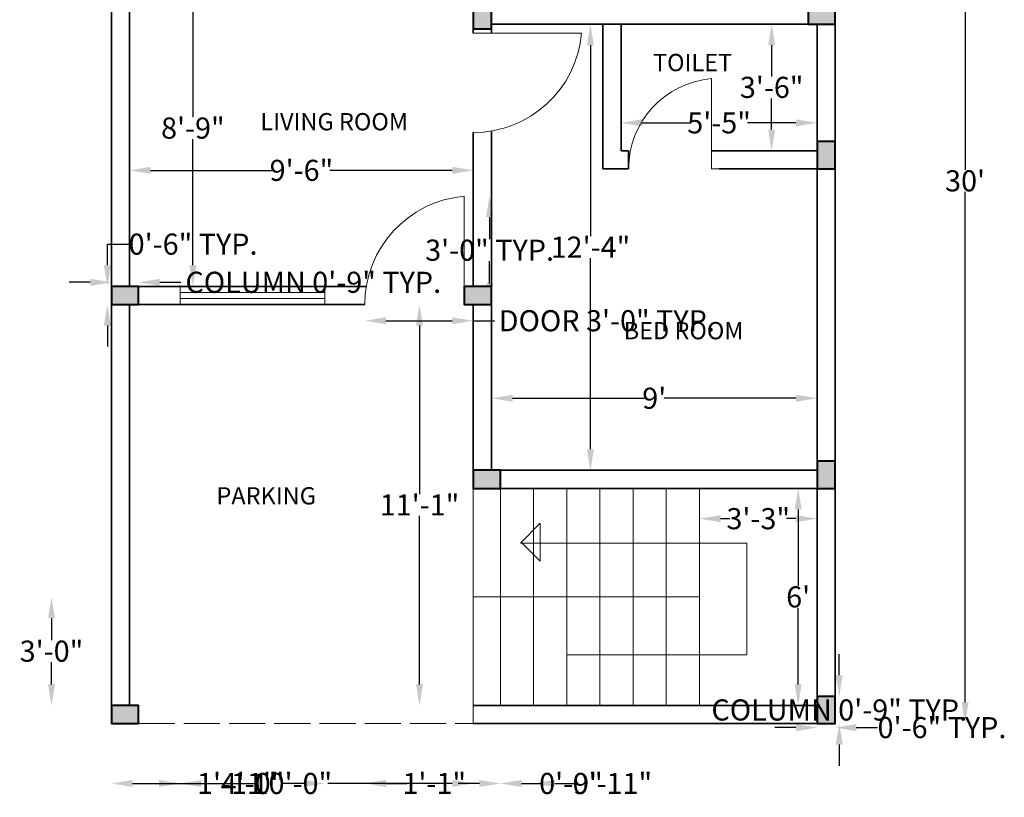
# Model space of a CAD drawing. Units: inches. Extents: x 2773 to 3100, y 2330 to 2750.
# Tile 1 of 2: x 2773 to 3100, y 2330 to 2588. Entities that reach past the tile are written whole.
import ezdxf

# ---------------------------------------------------------------- set-up
doc = ezdxf.new("R2010")
doc.units = ezdxf.units.IN
doc.linetypes.add('ACAD_ISO02W100', pattern=[15, 12, -3])
for name, color, linetype, lineweight in [('A-ANNO-DIMS', 2, 'Continuous', 18), ('A-AREA-IDEN', 7, 'Continuous', 18), ('A-COLS', 7, 'Continuous', 40), ('A-DOOR', 4, 'Continuous', 18), ('A-FLOR-PRKG', 7, 'ACAD_ISO02W100', 18), ('A-FLOR-STRS', 7, 'Continuous', 18), ('A-GLAZ', 4, 'Continuous', 18), ('A-WALL', 7, 'Continuous', 35)]:
    doc.layers.add(name, color=color, linetype=linetype, lineweight=lineweight)
doc.styles.get("Standard").update_dxf_attribs({"font": 'arial.ttf'})
doc.dimstyles.get("Standard").update_dxf_attribs({"dimtxt": 7, "dimasz": 7, "dimexe": 0.18, "dimexo": 0.0625, "dimgap": 0.09, "dimtad": 0, "dimtih": 1, "dimtoh": 1, "dimdec": 4, "dimzin": 0, "dimdsep": 46, "dimlunit": 4, "dimtxsty": 'Standard', "dimcen": 0.09, "dimse1": 1, "dimse2": 1, "dimadec": 0, "dimazin": 0, "dimtfac": 1, "dimtdec": 4, "dimtofl": 0, "dimtmove": 0, "dimatfit": 3, "dimfxl": 1, "dimtolj": 1, "dimtzin": 0, "dimarcsym": 0})

# ---------------------------------------------------------------- blocks, each defined once
blk = doc.blocks.new('*D7')
at = {"layer": 'A-ANNO-DIMS', "color": 0, "lineweight": -2, "transparency": 16777216}
for p, q in [((2979.63, 2553.92), (2995.73, 2553.92)), ((3030.63, 2553.92), (3014.52, 2553.92))]:
    blk.add_line(p, q, dxfattribs=at)
at = {"layer": 'A-ANNO-DIMS', "color": 0, "transparency": 16777216}
for points in [[(2979.63, 2555.09), (2979.63, 2552.76), (2972.63, 2553.92)], [(3030.63, 2555.09), (3030.63, 2552.76), (3037.63, 2553.92)]]:
    blk.add_solid(points, dxfattribs=at)
at = {"layer": 'Defpoints', "color": 0, "transparency": 16777216}
for p in [(2972.63, 2565.68), (3037.63, 2565.68), (3037.63, 2553.92)]:
    blk.add_point(p, dxfattribs=at)
at = {"layer": 'A-ANNO-DIMS', "color": 0, "transparency": 16777216, "insert": (3005.13, 2553.92), "char_height": 7, "attachment_point": 5}
blk.add_mtext('\\A1;5\'-5"', dxfattribs=at)
blk = doc.blocks.new('*D8')
at = {"layer": 'A-ANNO-DIMS', "color": 0, "lineweight": -2, "transparency": 16777216}
for p, q in [((3022.57, 2579.68), (3022.57, 2569.34)), ((3022.57, 2551.68), (3022.57, 2562.01))]:
    blk.add_line(p, q, dxfattribs=at)
at = {"layer": 'A-ANNO-DIMS', "color": 0, "transparency": 16777216}
for points in [[(3021.41, 2579.68), (3023.74, 2579.68), (3022.57, 2586.68)], [(3021.41, 2551.68), (3023.74, 2551.68), (3022.57, 2544.68)]]:
    blk.add_solid(points, dxfattribs=at)
at = {"layer": 'Defpoints', "color": 0, "transparency": 16777216}
for p in [(3022.92, 2586.68), (3022.57, 2544.68), (3022.92, 2544.68)]:
    blk.add_point(p, dxfattribs=at)
at = {"layer": 'A-ANNO-DIMS', "color": 0, "transparency": 16777216, "insert": (3022.57, 2565.68), "char_height": 7, "attachment_point": 5}
blk.add_mtext('\\A1;3\'-6"', dxfattribs=at)
blk = doc.blocks.new('*D9')
at = {"layer": 'A-ANNO-DIMS', "color": 0, "lineweight": -2, "transparency": 16777216}
for p, q in [((2962.47, 2579.68), (2962.47, 2516.28)), ((2962.47, 2445.68), (2962.47, 2509.07))]:
    blk.add_line(p, q, dxfattribs=at)
at = {"layer": 'A-ANNO-DIMS', "color": 0, "transparency": 16777216}
for points in [[(2961.3, 2579.68), (2963.63, 2579.68), (2962.47, 2586.68)], [(2961.3, 2445.68), (2963.63, 2445.68), (2962.47, 2438.68)]]:
    blk.add_solid(points, dxfattribs=at)
at = {"layer": 'Defpoints', "color": 0, "transparency": 16777216}
for p in [(2948, 2586.68), (2962.47, 2586.68), (2940.9, 2438.68)]:
    blk.add_point(p, dxfattribs=at)
at = {"layer": 'A-ANNO-DIMS', "color": 0, "transparency": 16777216, "insert": (2962.47, 2512.68), "char_height": 7, "attachment_point": 5}
blk.add_mtext('\\A1;12\'-4"', dxfattribs=at)
blk = doc.blocks.new('*D10')
at = {"layer": 'A-ANNO-DIMS', "color": 0, "lineweight": -2, "transparency": 16777216}
for p, q in [((2936.63, 2462.57), (2980.32, 2462.57)), ((3030.63, 2462.57), (2986.94, 2462.57))]:
    blk.add_line(p, q, dxfattribs=at)
at = {"layer": 'A-ANNO-DIMS', "color": 0, "transparency": 16777216}
for points in [[(2936.63, 2463.73), (2936.63, 2461.4), (2929.63, 2462.57)], [(3030.63, 2463.73), (3030.63, 2461.4), (3037.63, 2462.57)]]:
    blk.add_solid(points, dxfattribs=at)
at = {"layer": 'Defpoints', "color": 0, "transparency": 16777216}
for p in [(2929.63, 2525.39), (3037.63, 2525.39), (3037.63, 2462.57)]:
    blk.add_point(p, dxfattribs=at)
at = {"layer": 'A-ANNO-DIMS', "color": 0, "transparency": 16777216, "insert": (2983.63, 2462.57), "char_height": 7, "attachment_point": 5}
blk.add_mtext("\\A1;9'", dxfattribs=at)
blk = doc.blocks.new('*D12')
at = {"layer": 'A-ANNO-DIMS', "color": 0, "lineweight": -2, "transparency": 16777216}
for p, q in [((2830.63, 2597.68), (2830.63, 2555.84)), ((2830.63, 2506.68), (2830.63, 2548.51))]:
    blk.add_line(p, q, dxfattribs=at)
at = {"layer": 'A-ANNO-DIMS', "color": 0, "transparency": 16777216}
for points in [[(2829.47, 2597.68), (2831.8, 2597.68), (2830.63, 2604.68)], [(2829.47, 2506.68), (2831.8, 2506.68), (2830.63, 2499.68)]]:
    blk.add_solid(points, dxfattribs=at)
at = {"layer": 'Defpoints', "color": 0, "transparency": 16777216}
for p in [(2829.2, 2604.68), (2829.2, 2499.68), (2830.63, 2499.68)]:
    blk.add_point(p, dxfattribs=at)
at = {"layer": 'A-ANNO-DIMS', "color": 0, "transparency": 16777216, "insert": (2830.63, 2552.18), "char_height": 7, "attachment_point": 5}
blk.add_mtext('\\A1;8\'-9"', dxfattribs=at)
blk = doc.blocks.new('*D13')
at = {"layer": 'A-ANNO-DIMS', "color": 0, "lineweight": -2, "transparency": 16777216}
for p, q in [((2816.63, 2538.16), (2857.23, 2538.16)), ((2916.63, 2538.16), (2876.02, 2538.16))]:
    blk.add_line(p, q, dxfattribs=at)
at = {"layer": 'A-ANNO-DIMS', "color": 0, "transparency": 16777216}
for points in [[(2816.63, 2539.33), (2816.63, 2537), (2809.63, 2538.16)], [(2916.63, 2539.33), (2916.63, 2537), (2923.63, 2538.16)]]:
    blk.add_solid(points, dxfattribs=at)
at = {"layer": 'Defpoints', "color": 0, "transparency": 16777216}
for p in [(2923.63, 2538.16), (2809.63, 2530.09), (2923.63, 2530.09)]:
    blk.add_point(p, dxfattribs=at)
at = {"layer": 'A-ANNO-DIMS', "color": 0, "transparency": 16777216, "insert": (2866.63, 2538.16), "char_height": 7, "attachment_point": 5}
blk.add_mtext('\\A1;9\'-6"', dxfattribs=at)
blk = doc.blocks.new('*D14')
at = {"layer": 'A-ANNO-DIMS', "color": 0, "lineweight": -2, "transparency": 16777216}
for p, q in [((2905.79, 2486.68), (2905.79, 2430.78)), ((2905.79, 2367.68), (2905.79, 2423.57))]:
    blk.add_line(p, q, dxfattribs=at)
at = {"layer": 'A-ANNO-DIMS', "color": 0, "transparency": 16777216}
for points in [[(2904.63, 2486.68), (2906.96, 2486.68), (2905.79, 2493.68)], [(2904.63, 2367.68), (2906.96, 2367.68), (2905.79, 2360.68)]]:
    blk.add_solid(points, dxfattribs=at)
at = {"layer": 'Defpoints', "color": 0, "transparency": 16777216}
for p in [(2820.04, 2493.68), (2820.04, 2360.68), (2905.79, 2360.68)]:
    blk.add_point(p, dxfattribs=at)
at = {"layer": 'A-ANNO-DIMS', "color": 0, "transparency": 16777216, "insert": (2905.79, 2427.18), "char_height": 7, "attachment_point": 5}
blk.add_mtext('\\A1;11\'-1"', dxfattribs=at)
blk = doc.blocks.new('*D16')
at = {"layer": 'A-ANNO-DIMS', "color": 0, "lineweight": -2, "transparency": 16777216}
for p, q in [((3086.7, 2707.68), (3086.7, 2538.34)), ((3086.7, 2361.68), (3086.7, 2531.01))]:
    blk.add_line(p, q, dxfattribs=at)
at = {"layer": 'A-ANNO-DIMS', "color": 0, "transparency": 16777216}
for points in [[(3085.54, 2707.68), (3087.87, 2707.68), (3086.7, 2714.68)], [(3085.54, 2361.68), (3087.87, 2361.68), (3086.7, 2354.68)]]:
    blk.add_solid(points, dxfattribs=at)
at = {"layer": 'Defpoints', "color": 0, "transparency": 16777216}
for p in [(3043.63, 2714.68), (3043.63, 2354.68), (3086.7, 2354.68)]:
    blk.add_point(p, dxfattribs=at)
at = {"layer": 'A-ANNO-DIMS', "color": 0, "transparency": 16777216, "insert": (3086.7, 2534.68), "char_height": 7, "attachment_point": 5}
blk.add_mtext("\\A1;30'", dxfattribs=at)
blk = doc.blocks.new('*D17')
at = {"layer": 'A-ANNO-DIMS', "color": 0, "lineweight": -2, "transparency": 16777216}
for p, q in [((3031.36, 2425.68), (3031.36, 2400.34)), ((3031.36, 2367.68), (3031.36, 2393.01))]:
    blk.add_line(p, q, dxfattribs=at)
at = {"layer": 'A-ANNO-DIMS', "color": 0, "transparency": 16777216}
for points in [[(3030.19, 2425.68), (3032.52, 2425.68), (3031.36, 2432.68)], [(3030.19, 2367.68), (3032.52, 2367.68), (3031.36, 2360.68)]]:
    blk.add_solid(points, dxfattribs=at)
at = {"layer": 'Defpoints', "color": 0, "transparency": 16777216}
for p in [(2998.63, 2432.68), (2998.63, 2360.68), (3031.36, 2360.68)]:
    blk.add_point(p, dxfattribs=at)
at = {"layer": 'A-ANNO-DIMS', "color": 0, "transparency": 16777216, "insert": (3031.36, 2396.68), "char_height": 7, "attachment_point": 5}
blk.add_mtext("\\A1;6'", dxfattribs=at)
blk = doc.blocks.new('*D18')
at = {"layer": 'A-ANNO-DIMS', "color": 0, "lineweight": -2, "transparency": 16777216}
for p, q in [((3005.63, 2422.63), (3008.74, 2422.63)), ((3030.63, 2422.63), (3027.52, 2422.63))]:
    blk.add_line(p, q, dxfattribs=at)
at = {"layer": 'A-ANNO-DIMS', "color": 0, "transparency": 16777216}
for points in [[(3005.63, 2423.79), (3005.63, 2421.46), (2998.63, 2422.63)], [(3030.63, 2423.79), (3030.63, 2421.46), (3037.63, 2422.63)]]:
    blk.add_solid(points, dxfattribs=at)
at = {"layer": 'Defpoints', "color": 0, "transparency": 16777216}
for p in [(2998.63, 2432.68), (3037.63, 2432.68), (3037.63, 2422.63)]:
    blk.add_point(p, dxfattribs=at)
at = {"layer": 'A-ANNO-DIMS', "color": 0, "transparency": 16777216, "insert": (3018.13, 2422.63), "char_height": 7, "attachment_point": 5}
blk.add_mtext('\\A1;3\'-3"', dxfattribs=at)
blk = doc.blocks.new('COL-9X6')
h = blk.add_hatch(color=256)
h.dxf.hatch_style = 1
h.paths.add_polyline_path([(0, 6), (0, 0), (9, 0), (9, 6)])
blk.add_lwpolyline([(9, 0), (9, 6), (0, 6), (0, 0)], close=True)
blk = doc.blocks.new('COL-6X9')
h = blk.add_hatch(color=256)
h.dxf.hatch_style = 1
h.paths.add_polyline_path([(6, 9), (0, 9), (0, 0), (6, 0)])
blk.add_lwpolyline([(6, 9), (0, 9), (0, 0), (6, 0)], close=True)
blk = doc.blocks.new('DOOR-SWING-30')
for p, q in [((-2.5, 29.9), (-2.5, 0)), ((0, 0), (-2.5, 0)), ((-2.5, 0), (0, 0))]:
    blk.add_line(p, q)
blk.add_arc((0, 0), 30, 94.7802, 180)
blk = doc.blocks.new('DOOR-SWING-36')
for p, q in [((0, 6), (0, 36)), ((0, 36), (0, 6)), ((-3, 35.87), (-3, 0))]:
    blk.add_line(p, q)
blk.add_arc((0, 0), 36, 94.7802, 180)
blk = doc.blocks.new('*D23')
at = {"layer": 'A-ANNO-DIMS', "color": 0, "lineweight": -2, "transparency": 16777216}
for p, q in [((2796.63, 2501.03), (2789.63, 2501.03)), ((2819.63, 2501.03), (2826.63, 2501.03))]:
    blk.add_line(p, q, dxfattribs=at)
at = {"layer": 'A-ANNO-DIMS', "color": 0, "transparency": 16777216}
for points in [[(2796.63, 2502.19), (2796.63, 2499.86), (2803.63, 2501.03)], [(2819.63, 2502.19), (2819.63, 2499.86), (2812.63, 2501.03)]]:
    blk.add_solid(points, dxfattribs=at)
at = {"layer": 'Defpoints', "color": 0, "transparency": 16777216}
for p in [(2803.63, 2499.68), (2812.63, 2501.03), (2812.63, 2499.68)]:
    blk.add_point(p, dxfattribs=at)
at = {"layer": 'A-ANNO-DIMS', "color": 0, "transparency": 16777216, "insert": (2870.56, 2501.03), "char_height": 7, "attachment_point": 5}
blk.add_mtext('\\A1;COLUMN 0\'-9" TYP.', dxfattribs=at)
blk = doc.blocks.new('*D24')
at = {"layer": 'A-ANNO-DIMS', "color": 0, "lineweight": -2, "transparency": 16777216}
for p, q in [((2802.28, 2506.68), (2802.28, 2513.68)), ((2802.28, 2513.68), (2809.28, 2513.68)), ((2802.28, 2486.68), (2802.28, 2479.68))]:
    blk.add_line(p, q, dxfattribs=at)
at = {"layer": 'A-ANNO-DIMS', "color": 0, "transparency": 16777216}
for points in [[(2801.11, 2506.68), (2803.44, 2506.68), (2802.28, 2499.68)], [(2801.11, 2486.68), (2803.44, 2486.68), (2802.28, 2493.68)]]:
    blk.add_solid(points, dxfattribs=at)
at = {"layer": 'Defpoints', "color": 0, "transparency": 16777216}
for p in [(2802.28, 2499.68), (2803.63, 2499.68), (2803.63, 2493.68)]:
    blk.add_point(p, dxfattribs=at)
at = {"layer": 'A-ANNO-DIMS', "color": 0, "transparency": 16777216, "insert": (2830.7, 2513.68), "char_height": 7, "attachment_point": 5}
blk.add_mtext('\\A1;0\'-6" TYP.', dxfattribs=at)
blk = doc.blocks.new('*D25')
at = {"layer": 'A-ANNO-DIMS', "color": 0, "lineweight": -2, "transparency": 16777216}
for p, q in [((3044.98, 2370.68), (3044.98, 2377.68)), ((3044.98, 2347.68), (3044.98, 2340.68))]:
    blk.add_line(p, q, dxfattribs=at)
at = {"layer": 'A-ANNO-DIMS', "color": 0, "transparency": 16777216}
for points in [[(3043.81, 2370.68), (3046.14, 2370.68), (3044.98, 2363.68)], [(3043.81, 2347.68), (3046.14, 2347.68), (3044.98, 2354.68)]]:
    blk.add_solid(points, dxfattribs=at)
at = {"layer": 'Defpoints', "color": 0, "transparency": 16777216}
for p in [(3043.63, 2363.68), (3044.98, 2363.68), (3043.63, 2354.68)]:
    blk.add_point(p, dxfattribs=at)
at = {"layer": 'A-ANNO-DIMS', "color": 0, "transparency": 16777216, "insert": (3044.98, 2359.18), "char_height": 7, "attachment_point": 5}
blk.add_mtext('\\A1;COLUMN 0\'-9" TYP.', dxfattribs=at)
blk = doc.blocks.new('*D26')
at = {"layer": 'A-ANNO-DIMS', "color": 0, "lineweight": -2, "transparency": 16777216}
for p, q in [((3030.63, 2353.33), (3023.63, 2353.33)), ((3050.63, 2353.33), (3057.63, 2353.33))]:
    blk.add_line(p, q, dxfattribs=at)
at = {"layer": 'A-ANNO-DIMS', "color": 0, "transparency": 16777216}
for points in [[(3030.63, 2354.49), (3030.63, 2352.16), (3037.63, 2353.33)], [(3050.63, 2354.49), (3050.63, 2352.16), (3043.63, 2353.33)]]:
    blk.add_solid(points, dxfattribs=at)
at = {"layer": 'Defpoints', "color": 0, "transparency": 16777216}
for p in [(3037.63, 2354.68), (3043.63, 2354.68), (3043.63, 2353.33)]:
    blk.add_point(p, dxfattribs=at)
at = {"layer": 'A-ANNO-DIMS', "color": 0, "transparency": 16777216, "insert": (3079.05, 2353.33), "char_height": 7, "attachment_point": 5}
blk.add_mtext('\\A1;0\'-6" TYP.', dxfattribs=at)
blk = doc.blocks.new('*D29')
at = {"layer": 'A-ANNO-DIMS', "color": 0, "lineweight": -2, "transparency": 16777216}
for p, q in [((2894.63, 2488.28), (2916.63, 2488.28)), ((2923.63, 2488.28), (2930.63, 2488.28))]:
    blk.add_line(p, q, dxfattribs=at)
at = {"layer": 'A-ANNO-DIMS', "color": 0, "transparency": 16777216}
for points in [[(2894.63, 2489.44), (2894.63, 2487.11), (2887.63, 2488.28)], [(2916.63, 2489.44), (2916.63, 2487.11), (2923.63, 2488.28)]]:
    blk.add_solid(points, dxfattribs=at)
at = {"layer": 'Defpoints', "color": 0, "transparency": 16777216}
for p in [(2887.63, 2493.68), (2923.63, 2493.68), (2923.63, 2488.28)]:
    blk.add_point(p, dxfattribs=at)
at = {"layer": 'A-ANNO-DIMS', "color": 0, "transparency": 16777216, "insert": (2967.9, 2488.28), "char_height": 7, "attachment_point": 5}
blk.add_mtext('\\A1;DOOR 3\'-0" TYP.', dxfattribs=at)
blk = doc.blocks.new('*D30')
at = {"layer": 'A-ANNO-DIMS', "color": 0, "lineweight": -2, "transparency": 16777216}
for p, q in [((2929.03, 2522.68), (2929.03, 2515.34)), ((2929.03, 2500.68), (2929.03, 2508.01))]:
    blk.add_line(p, q, dxfattribs=at)
at = {"layer": 'A-ANNO-DIMS', "color": 0, "transparency": 16777216}
for points in [[(2927.86, 2522.68), (2930.19, 2522.68), (2929.03, 2529.68)], [(2927.86, 2500.68), (2930.19, 2500.68), (2929.03, 2493.68)]]:
    blk.add_solid(points, dxfattribs=at)
at = {"layer": 'Defpoints', "color": 0, "transparency": 16777216}
for p in [(2923.63, 2529.68), (2929.03, 2529.68), (2923.63, 2493.68)]:
    blk.add_point(p, dxfattribs=at)
at = {"layer": 'A-ANNO-DIMS', "color": 0, "transparency": 16777216, "insert": (2929.03, 2511.68), "char_height": 7, "attachment_point": 5}
blk.add_mtext('\\A1;3\'-0" TYP.', dxfattribs=at)
blk = doc.blocks.new('*D31')
at = {"layer": 'A-ANNO-DIMS', "color": 0, "lineweight": -2, "transparency": 16777216}
for p, q in [((2810.63, 2334.8), (2819.41, 2334.8)), ((2826.41, 2334.8), (2833.41, 2334.8))]:
    blk.add_line(p, q, dxfattribs=at)
at = {"layer": 'A-ANNO-DIMS', "color": 0, "transparency": 16777216}
for points in [[(2810.63, 2335.97), (2810.63, 2333.64), (2803.63, 2334.8)], [(2819.41, 2335.97), (2819.41, 2333.64), (2826.41, 2334.8)]]:
    blk.add_solid(points, dxfattribs=at)
at = {"layer": 'Defpoints', "color": 0, "transparency": 16777216}
for p in [(2803.63, 2493.68), (2826.41, 2493.68), (2826.41, 2334.8)]:
    blk.add_point(p, dxfattribs=at)
at = {"layer": 'A-ANNO-DIMS', "color": 0, "transparency": 16777216, "insert": (2845.2, 2334.8), "char_height": 7, "attachment_point": 5}
blk.add_mtext('\\A1;1\'-11"', dxfattribs=at)
blk = doc.blocks.new('*D32')
at = {"layer": 'A-ANNO-DIMS', "color": 0, "lineweight": -2, "transparency": 16777216}
for p, q in [((2833.41, 2334.8), (2840.88, 2334.8)), ((2867.41, 2334.8), (2859.95, 2334.8))]:
    blk.add_line(p, q, dxfattribs=at)
at = {"layer": 'A-ANNO-DIMS', "color": 0, "transparency": 16777216}
for points in [[(2833.41, 2335.97), (2833.41, 2333.64), (2826.41, 2334.8)], [(2867.41, 2335.97), (2867.41, 2333.64), (2874.41, 2334.8)]]:
    blk.add_solid(points, dxfattribs=at)
at = {"layer": 'Defpoints', "color": 0, "transparency": 16777216}
for p in [(2826.41, 2493.68), (2874.41, 2493.68), (2874.41, 2334.8)]:
    blk.add_point(p, dxfattribs=at)
at = {"layer": 'A-ANNO-DIMS', "color": 0, "transparency": 16777216, "insert": (2850.41, 2334.8), "char_height": 7, "attachment_point": 5}
blk.add_mtext('\\A1;4\'-0"', dxfattribs=at)
blk = doc.blocks.new('*D33')
at = {"layer": 'A-ANNO-DIMS', "color": 0, "lineweight": -2, "transparency": 16777216}
for p, q in [((2867.41, 2334.8), (2860.41, 2334.8)), ((2894.63, 2334.8), (2901.63, 2334.8))]:
    blk.add_line(p, q, dxfattribs=at)
at = {"layer": 'A-ANNO-DIMS', "color": 0, "transparency": 16777216}
for points in [[(2867.41, 2335.97), (2867.41, 2333.64), (2874.41, 2334.8)], [(2894.63, 2335.97), (2894.63, 2333.64), (2887.63, 2334.8)]]:
    blk.add_solid(points, dxfattribs=at)
at = {"layer": 'Defpoints', "color": 0, "transparency": 16777216}
for p in [(2874.41, 2493.68), (2887.63, 2493.68), (2887.63, 2334.8)]:
    blk.add_point(p, dxfattribs=at)
at = {"layer": 'A-ANNO-DIMS', "color": 0, "transparency": 16777216, "insert": (2910.69, 2334.8), "char_height": 7, "attachment_point": 5}
blk.add_mtext('\\A1;1\'-1"', dxfattribs=at)
blk = doc.blocks.new('*D34')
at = {"layer": 'A-ANNO-DIMS', "color": 0, "lineweight": -2, "transparency": 16777216}
for p, q in [((2810.63, 2334.8), (2851.84, 2334.8)), ((2916.63, 2334.8), (2875.41, 2334.8))]:
    blk.add_line(p, q, dxfattribs=at)
at = {"layer": 'A-ANNO-DIMS', "color": 0, "transparency": 16777216}
for points in [[(2810.63, 2335.97), (2810.63, 2333.64), (2803.63, 2334.8)], [(2916.63, 2335.97), (2916.63, 2333.64), (2923.63, 2334.8)]]:
    blk.add_solid(points, dxfattribs=at)
at = {"layer": 'Defpoints', "color": 0, "transparency": 16777216}
for p in [(2803.63, 2354.68), (2923.63, 2354.68), (2923.63, 2334.8)]:
    blk.add_point(p, dxfattribs=at)
at = {"layer": 'A-ANNO-DIMS', "color": 0, "transparency": 16777216, "insert": (2863.63, 2334.8), "char_height": 7, "attachment_point": 5}
blk.add_mtext('\\A1;10\'-0"', dxfattribs=at)
blk = doc.blocks.new('*D35')
at = {"layer": 'A-ANNO-DIMS', "color": 0, "lineweight": -2, "transparency": 16777216}
for p, q in [((2925.63, 2334.8), (2918.63, 2334.8)), ((2950.63, 2334.8), (2957.63, 2334.8))]:
    blk.add_line(p, q, dxfattribs=at)
at = {"layer": 'A-ANNO-DIMS', "color": 0, "transparency": 16777216}
for points in [[(2925.63, 2335.97), (2925.63, 2333.64), (2932.63, 2334.8)], [(2950.63, 2335.97), (2950.63, 2333.64), (2943.63, 2334.8)]]:
    blk.add_solid(points, dxfattribs=at)
at = {"layer": 'Defpoints', "color": 0, "transparency": 16777216}
for p in [(2932.63, 2360.68), (2943.63, 2360.68), (2943.63, 2334.8)]:
    blk.add_point(p, dxfattribs=at)
at = {"layer": 'A-ANNO-DIMS', "color": 0, "transparency": 16777216, "insert": (2969.74, 2334.8), "char_height": 7, "attachment_point": 5}
blk.add_mtext('\\A1;0\'-11"', dxfattribs=at)
blk = doc.blocks.new('*D36')
at = {"layer": 'A-ANNO-DIMS', "color": 0, "lineweight": -2, "transparency": 16777216}
for p, q in [((2783.75, 2389.68), (2783.75, 2382.34)), ((2783.75, 2367.68), (2783.75, 2375.01))]:
    blk.add_line(p, q, dxfattribs=at)
at = {"layer": 'A-ANNO-DIMS', "color": 0, "transparency": 16777216}
for points in [[(2782.59, 2389.68), (2784.92, 2389.68), (2783.75, 2396.68)], [(2782.59, 2367.68), (2784.92, 2367.68), (2783.75, 2360.68)]]:
    blk.add_solid(points, dxfattribs=at)
at = {"layer": 'Defpoints', "color": 0, "transparency": 16777216}
for p in [(2783.75, 2396.68), (2923.63, 2396.68), (2923.63, 2360.68)]:
    blk.add_point(p, dxfattribs=at)
at = {"layer": 'A-ANNO-DIMS', "color": 0, "transparency": 16777216, "insert": (2783.75, 2378.68), "char_height": 7, "attachment_point": 5}
blk.add_mtext('\\A1;3\'-0"', dxfattribs=at)
blk = doc.blocks.new('*D37')
at = {"layer": 'A-ANNO-DIMS', "color": 0, "lineweight": -2, "transparency": 16777216}
for p, q in [((2916.63, 2334.8), (2909.63, 2334.8)), ((2939.63, 2334.8), (2946.63, 2334.8))]:
    blk.add_line(p, q, dxfattribs=at)
at = {"layer": 'A-ANNO-DIMS', "color": 0, "transparency": 16777216}
for points in [[(2916.63, 2335.97), (2916.63, 2333.64), (2923.63, 2334.8)], [(2939.63, 2335.97), (2939.63, 2333.64), (2932.63, 2334.8)]]:
    blk.add_solid(points, dxfattribs=at)
at = {"layer": 'Defpoints', "color": 0, "transparency": 16777216}
for p in [(2923.63, 2360.68), (2932.63, 2360.68), (2932.63, 2334.8)]:
    blk.add_point(p, dxfattribs=at)
at = {"layer": 'A-ANNO-DIMS', "color": 0, "transparency": 16777216, "insert": (2956.02, 2334.8), "char_height": 7, "attachment_point": 5}
blk.add_mtext('\\A1;0\'-9"', dxfattribs=at)
blk = doc.blocks.new('*D38')
at = {"layer": 'A-ANNO-DIMS', "color": 0, "lineweight": -2, "transparency": 16777216}
for p, q in [((2930.63, 2734.55), (2951.71, 2734.55)), ((2991.63, 2734.55), (2970.54, 2734.55))]:
    blk.add_line(p, q, dxfattribs=at)
at = {"layer": 'A-ANNO-DIMS', "color": 0, "transparency": 16777216}
for points in [[(2930.63, 2735.72), (2930.63, 2733.39), (2923.63, 2734.55)], [(2991.63, 2735.72), (2991.63, 2733.39), (2998.63, 2734.55)]]:
    blk.add_solid(points, dxfattribs=at)
at = {"layer": 'Defpoints', "color": 0, "transparency": 16777216}
for p in [(2998.63, 2734.55), (2923.63, 2432.68), (2998.63, 2432.68)]:
    blk.add_point(p, dxfattribs=at)
at = {"layer": 'A-ANNO-DIMS', "color": 0, "transparency": 16777216, "insert": (2961.13, 2734.55), "char_height": 7, "attachment_point": 5}
blk.add_mtext('\\A1;6\'-3"', dxfattribs=at)

msp = doc.modelspace()

# ---------------------------------------------------------------- linework, layer by layer
at = {"layer": 'A-DOOR'}
for p, q in [((2923.62737, 2586.67688), (2923.62737, 2583.67688)), ((2923.62737, 2583.67688), (2923.62737, 2586.67688)), ((2923.62737, 2493.67688), (2920.62737, 2493.67688)), ((2920.62737, 2493.67688), (2923.62737, 2493.67688)), ((2920.62737, 2493.67688), (2923.62737, 2493.67688))]:
    msp.add_line(p, q, dxfattribs=at)
at = {"layer": 'A-FLOR-PRKG'}
msp.add_line((2812.62737, 2354.67688), (2923.62737, 2354.67688), dxfattribs=at)
at = {"layer": 'A-FLOR-STRS'}
for p, q in [((2923.62737, 2354.67688), (2923.62737, 2432.67688)), ((2932.62737, 2360.67688), (2932.62737, 2432.67688)), ((2943.62737, 2360.67688), (2943.62737, 2432.67688)), ((2954.62737, 2360.67688), (2954.62737, 2432.67688)), ((2965.62737, 2360.67688), (2965.62737, 2432.67688)), ((2976.62737, 2360.67688), (2976.62737, 2432.67688)), ((2987.62737, 2360.67688), (2987.62737, 2432.67688)), ((2998.62737, 2360.67688), (2998.62737, 2432.67688)), ((2939.29782, 2414.53548), (2945.84469, 2421.08234)), ((2945.84469, 2421.08234), (2945.84469, 2408.47924)), ((3014.36176, 2414.53548), (2939.29782, 2414.53548)), ((2945.84469, 2408.47924), (2939.54314, 2414.78079)), ((3014.36176, 2377.41658), (3014.36176, 2414.53548)), ((2998.62737, 2396.67688), (2923.62737, 2396.67688)), ((2954.62737, 2377.41658), (3014.36176, 2377.41658))]:
    msp.add_line(p, q, dxfattribs=at)
at = {"layer": 'A-GLAZ'}
for p, q in [((2826.4137, 2499.67688), (2874.4137, 2499.67688)), ((2826.4137, 2493.67688), (2826.4137, 2499.67688)), ((2874.4137, 2499.67688), (2874.4137, 2493.67688)), ((2826.4137, 2497.67688), (2874.4137, 2497.67688)), ((2826.4137, 2495.67688), (2874.4137, 2495.67688)), ((2874.4137, 2493.67688), (2826.4137, 2493.67688))]:
    msp.add_line(p, q, dxfattribs=at)
at = {"layer": 'A-WALL'}
for p, q in [((2803.62737, 2714.67688), (2803.62737, 2354.67688)), ((3043.62737, 2354.67688), (3043.62737, 2714.67688)), ((2809.62737, 2708.67688), (2809.62737, 2499.67688)), ((2923.62737, 2595.67688), (2923.62737, 2583.67688)), ((2929.62737, 2586.67688), (3037.62737, 2586.67688)), ((2929.62737, 2586.67688), (2929.62737, 2583.67688)), ((2966.62737, 2544.67688), (2966.62737, 2586.67688)), ((2972.62737, 2544.67688), (2972.62737, 2586.67688)), ((3037.62737, 2544.67688), (3037.62737, 2586.67688)), ((2923.62737, 2550.67688), (2923.62737, 2499.67688)), ((2929.62737, 2551.1804), (2929.62737, 2438.67688)), ((2966.62737, 2538.67688), (2966.62737, 2544.67688)), ((2972.62737, 2544.67688), (2975.12737, 2544.67688)), ((2975.12737, 2544.67688), (2972.62737, 2544.67688)), ((2975.12737, 2538.67688), (2975.12737, 2544.67688)), ((3005.12737, 2544.67688), (3002.62737, 2544.67688)), ((3037.62737, 2544.67688), (3005.12737, 2544.67688)), ((3005.12737, 2544.67688), (3037.62737, 2544.67688)), ((2975.12737, 2538.67688), (2966.62737, 2538.67688)), ((2972.62737, 2538.67688), (2975.12737, 2538.67688)), ((3037.62737, 2538.67688), (3005.12737, 2538.67688)), ((3005.12737, 2538.67688), (3037.62737, 2538.67688)), ((3037.62737, 2438.67688), (3037.62737, 2538.67688)), ((2809.62737, 2499.67688), (2888.13089, 2499.67688)), ((2920.62737, 2499.67688), (2923.62737, 2499.67688)), ((2809.62737, 2493.67688), (2887.62737, 2493.67688)), ((2809.62737, 2493.67688), (2809.62737, 2360.67688)), ((2923.62737, 2493.67688), (2923.62737, 2432.67688)), ((2929.62737, 2438.67688), (3037.62737, 2438.67688)), ((2929.62737, 2432.67688), (2923.62737, 2432.67688)), ((2929.62737, 2432.67688), (3037.62737, 2432.67688)), ((3037.62737, 2360.67688), (3037.62737, 2432.67688)), ((2809.62737, 2360.67688), (2812.62737, 2360.67688)), ((2923.62737, 2360.67688), (2929.62737, 2360.67688)), ((2929.62737, 2360.67688), (3037.62737, 2360.67688)), ((2923.62737, 2354.67688), (3043.62737, 2354.67688))]:
    msp.add_line(p, q, dxfattribs=at)

# ---------------------------------------------------------------- block references
at = {"layer": 'A-COLS', "rotation": 89.99999999999864}
msp.add_blockref('COL-9X6', (2929.62737, 2585.08543), dxfattribs=at)
at = {"layer": 'A-COLS'}
for name, p in [('COL-9X6', (3034.62737, 2586.67688)), ('COL-6X9', (3037.62737, 2538.67688)), ('COL-9X6', (2803.62737, 2493.67688)), ('COL-9X6', (2920.62737, 2493.67634)), ('COL-6X9', (3037.62737, 2432.67688)), ('COL-9X6', (2923.62737, 2432.67688)), ('COL-6X9', (3037.62737, 2354.67688)), ('COL-9X6', (2803.62737, 2354.67688))]:
    msp.add_blockref(name, p, dxfattribs=at)
at = {"layer": 'A-DOOR', "extrusion": (0, 0, -1), "zscale": -1, "rotation": 90.00000000000136}
msp.add_blockref('DOOR-SWING-36', (-2923.62737, 2586.67688), dxfattribs=at)
at = {"layer": 'A-DOOR'}
for name, p in [('DOOR-SWING-30', (3005.12737, 2538.67688)), ('DOOR-SWING-36', (2923.62737, 2493.67688))]:
    msp.add_blockref(name, p, dxfattribs=at)

# ---------------------------------------------------------------- texts
at = {"layer": 'A-AREA-IDEN', "attachment_point": 1}
for s, insert, char_height in [('TOILET', (2983.20972, 2576.77525), 5.720006), ('LIVING ROOM', (2853.0113, 2557.15696), 5.7200058), ('BED ROOM', (2973.49824, 2487.84762), 5.720006), ('PARKING', (2838.45346, 2433.07145), 5.720006)]:
    msp.add_mtext_dynamic_manual_height_columns(s, width=353.6359827, gutter_width=28.60003, heights=[0], dxfattribs=dict(at, insert=insert, char_height=char_height))

# ---------------------------------------------------------------- dimensions: what is measured, and where the dimension line sits
at = {"layer": 'A-ANNO-DIMS'}
for base, p1, p2, override, picture, middle in [((2998.62737, 2734.55188), (2923.62737, 2432.67688), (2998.62737, 2432.67688), {"dimdec": 1, "dimlfac": 1, "dimrnd": 0, "dimzin": 1, "dimdsep": 46, "dimlunit": 4, "dimfrac": 2}, '*D38', (2961.12737, 2734.55188)), ((3037.62737, 2553.92397), (2972.62737, 2565.67688), (3037.62737, 2565.67688), {"dimclrd": 0, "dimclre": 0, "dimclrt": 0}, '*D7', (3005.12737, 2553.92397)), ((2923.62737, 2538.1628), (2809.62737, 2530.08584), (2923.62737, 2530.08584), {"dimclrd": 0, "dimclre": 0, "dimclrt": 0}, '*D13', (2866.62737, 2538.1628)), ((3037.62737, 2462.56626), (2929.62737, 2525.39278), (3037.62737, 2525.39278), {"dimclrd": 0, "dimclre": 0, "dimclrt": 0}, '*D10', (2983.62737, 2462.56626)), ((2826.4137, 2334.80188), (2803.62737, 2493.67688), (2826.4137, 2493.67688), {"dimdec": 1, "dimlfac": 1, "dimrnd": 0, "dimzin": 1, "dimdsep": 46, "dimlunit": 4, "dimfrac": 2}, '*D31', (2845.19743, 2334.80188)), ((2874.4137, 2334.80188), (2826.4137, 2493.67688), (2874.4137, 2493.67688), {"dimdec": 1, "dimlfac": 1, "dimrnd": 0, "dimzin": 1, "dimdsep": 46, "dimlunit": 4, "dimfrac": 2}, '*D32', (2850.4137, 2334.80188)), ((2887.62737, 2334.80188), (2874.4137, 2493.67688), (2887.62737, 2493.67688), {"dimdec": 1, "dimlfac": 1, "dimrnd": 0, "dimzin": 1, "dimdsep": 46, "dimlunit": 4, "dimfrac": 2}, '*D33', (2910.69179, 2334.80188)), ((3037.62737, 2422.62765), (2998.62737, 2432.67688), (3037.62737, 2432.67688), {"dimclrd": 0, "dimclre": 0, "dimclrt": 0}, '*D18', (3018.12737, 2422.62765)), ((2932.62737, 2334.80188), (2923.62737, 2360.67688), (2932.62737, 2360.67688), {"dimdec": 1, "dimlfac": 1, "dimrnd": 0, "dimzin": 1, "dimdsep": 46, "dimlunit": 4, "dimfrac": 2}, '*D37', (2956.02126, 2334.80188)), ((2943.62737, 2334.80188), (2932.62737, 2360.67688), (2943.62737, 2360.67688), {"dimdec": 1, "dimlfac": 1, "dimrnd": 0, "dimzin": 1, "dimdsep": 46, "dimlunit": 4, "dimfrac": 2}, '*D35', (2969.74056, 2334.80188)), ((2923.62737, 2334.80188), (2803.62737, 2354.67688), (2923.62737, 2354.67688), {"dimdec": 1, "dimlfac": 1, "dimrnd": 0, "dimzin": 1, "dimdsep": 46, "dimlunit": 4, "dimfrac": 2}, '*D34', (2863.62737, 2334.80188))]:
    dim = msp.add_linear_dim(base=base, p1=p1, p2=p2, dimstyle='Standard', override=override, dxfattribs=at)
    dim.commit()
    dim.dimension.update_dxf_attribs({"geometry": picture, "text_midpoint": middle})
for base, p1, p2, override, picture, middle in [((3086.70499, 2354.67688), (3043.62737, 2714.67688), (3043.62737, 2354.67688), {"dimclrd": 0, "dimclre": 0, "dimclrt": 0}, '*D16', (3086.70499, 2534.67688)), ((2830.63357, 2499.67688), (2829.20079, 2604.67688), (2829.20079, 2499.67688), {"dimclrd": 0, "dimclre": 0, "dimclrt": 0}, '*D12', (2830.63357, 2552.17688)), ((2962.46639, 2586.67688), (2940.898, 2438.67688), (2947.99978, 2586.67688), {"dimclrd": 0, "dimclre": 0, "dimclrt": 0}, '*D9', (2962.46639, 2512.67688)), ((3022.57431, 2544.67688), (3022.92109, 2586.67688), (3022.92109, 2544.67688), {"dimclrd": 0, "dimclre": 0, "dimclrt": 0}, '*D8', (3022.57431, 2565.67688)), ((2905.79281, 2360.67688), (2820.04475, 2493.67688), (2820.04475, 2360.67688), {"dimclrd": 0, "dimclre": 0, "dimclrt": 0}, '*D14', (2905.79281, 2427.17688)), ((3031.35647, 2360.67688), (2998.62737, 2432.67688), (2998.62737, 2360.67688), {"dimclrd": 0, "dimclre": 0, "dimclrt": 0}, '*D17', (3031.35647, 2396.67688)), ((2783.75237, 2396.67688), (2923.62737, 2360.67688), (2923.62737, 2396.67688), {"dimdec": 1, "dimlfac": 1, "dimrnd": 0, "dimzin": 1, "dimdsep": 46, "dimlunit": 4, "dimfrac": 2}, '*D36', (2783.75237, 2378.67688))]:
    dim = msp.add_linear_dim(base=base, p1=p1, p2=p2, angle=90, dimstyle='Standard', override=override, dxfattribs=at)
    dim.commit()
    dim.dimension.update_dxf_attribs({"geometry": picture, "text_midpoint": middle})
for base, p1, p2, text, picture, middle in [((2929.02737, 2529.67688), (2923.62737, 2493.67688), (2923.62737, 2529.67688), '<> TYP.', '*D30', (2929.02737, 2511.67688)), ((2802.27737, 2499.67688), (2803.62737, 2493.67688), (2803.62737, 2499.67688), '<> TYP.', '*D24', (2830.70161, 2513.67688)), ((3044.97737, 2363.67688), (3043.62737, 2354.67688), (3043.62737, 2363.67688), 'COLUMN <> TYP.', '*D25', (3044.97737, 2359.17688))]:
    dim = msp.add_linear_dim(base=base, p1=p1, p2=p2, angle=90, text=text, dimstyle='Standard', override={"dimdec": 1, "dimlfac": 1, "dimrnd": 0, "dimzin": 1, "dimdsep": 46, "dimlunit": 4, "dimfrac": 2}, dxfattribs=at)
    dim.commit()
    dim.dimension.update_dxf_attribs({"geometry": picture, "text_midpoint": middle})
for base, p1, p2, text, picture, middle in [((2812.62737, 2501.02688), (2803.62737, 2499.67688), (2812.62737, 2499.67688), 'COLUMN <> TYP.', '*D23', (2870.55809, 2501.02688)), ((2923.62737, 2488.27688), (2887.62737, 2493.67688), (2923.62737, 2493.67688), 'DOOR <> TYP.', '*D29', (2967.90427, 2488.27688)), ((3043.62737, 2353.32688), (3037.62737, 2354.67688), (3043.62737, 2354.67688), '<> TYP.', '*D26', (3079.05161, 2353.32688))]:
    dim = msp.add_linear_dim(base=base, p1=p1, p2=p2, text=text, dimstyle='Standard', override={"dimdec": 1, "dimlfac": 1, "dimrnd": 0, "dimzin": 1, "dimdsep": 46, "dimlunit": 4, "dimfrac": 2}, dxfattribs=at)
    dim.commit()
    dim.dimension.update_dxf_attribs({"geometry": picture, "text_midpoint": middle})

doc.saveas('drawing.dxf')
